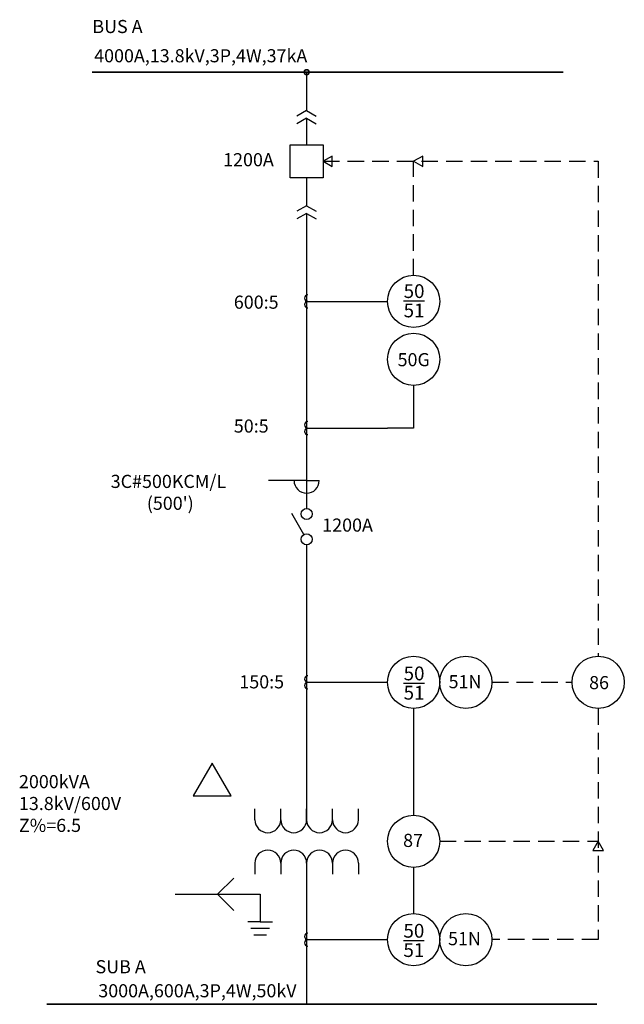
# Model space of a CAD drawing. Units: millimetres. Extents: x 325 to 734, y 204 to 452.
# Tile 1 of 1: x 642.1 to 734.2, y 301.6 to 451.7. Entities that reach past the tile are written whole.
import ezdxf

# ---------------------------------------------------------------- set-up
doc = ezdxf.new("R2010")
doc.units = ezdxf.units.MM
doc.header["$MEASUREMENT"] = 0
doc.linetypes.add('HIDDENX2', pattern=[0.75, 0.5, -0.25])
for name, color, linetype, lineweight in [('E-ANNO-TEXT', 7, 'Continuous', 25), ('E-CTRL-RLAY', 5, 'Continuous', 30), ('E-CTRL-SENS', 5, 'Continuous', 25), ('E-CTRL-SYMB', 3, 'Continuous', 30), ('E-CTRL-TRIP', 1, 'HIDDENX2', 30), ('E-POWR-BUSB', 3, 'Continuous', 35), ('E-POWR-CABL', 5, 'Continuous', 30), ('E-POWR-CONN', 7, 'Continuous', 30), ('E-POWR-CT', 5, 'Continuous', 30), ('E-POWR-FEED', 3, 'Continuous', 30), ('E-POWR-IDEN', 6, 'Continuous', 25), ('E-POWR-SWGR', 6, 'Continuous', 30), ('E-POWR-XFMR', 6, 'Continuous', 30)]:
    doc.layers.add(name, color=color, linetype=linetype, lineweight=lineweight)
doc.styles.get("Standard").update_dxf_attribs({"font": 'arial.ttf'})

# ---------------------------------------------------------------- blocks, each defined once
blk = doc.blocks.new('DRAWOUT-CONTACT')
for p, q in [((0, 0), (-1.47, -0.85)), ((0, 0), (1.47, -0.85)), ((0, -1.17), (-1.47, -2.01)), ((0, -1.17), (1.47, -2.01))]:
    blk.add_line(p, q)
blk = doc.blocks.new('XFMR-WINDING')
for p, q in [((-7.89, 0), (-7.89, 1.68)), ((-3.95, 0), (-3.95, 1.68)), ((0, 0), (0, 1.68)), ((3.95, 0), (3.95, 1.68)), ((7.89, 0), (7.89, 1.68))]:
    blk.add_line(p, q)
for centre in [(-5.92, 0), (-1.97, 0), (1.97, 0), (5.92, 0)]:
    blk.add_arc(centre, 1.97, 180, 0)
blk = doc.blocks.new('CURRENT-TRANSFORMER')
for centre in [(0.19, 0.5), (0.19, -0.5)]:
    blk.add_arc(centre, 0.501, 90, 270)
blk = doc.blocks.new('PROTECTIVE-RELAY')
blk.add_circle((0, 0), 3.98)
blk = doc.blocks.new('TRIP-ARROW')
blk.add_lwpolyline([(0.79, -1.38), (0, 0), (-0.79, -1.38)], close=True)

msp = doc.modelspace()

# ---------------------------------------------------------------- linework, layer by layer
at = {"layer": 'E-CTRL-SENS'}
for p, q in [((685.83, 408.77), (698.14, 408.77)), ((702.13, 395.94), (702.13, 389.45)), ((685.83, 389.45), (698.14, 389.45)), ((702.13, 389.45), (698.14, 389.45)), ((685.83, 350.69), (698.14, 350.69)), ((702.13, 346.71), (702.13, 330.42)), ((702.13, 322.45), (702.13, 315.44)), ((685.83, 311.45), (698.14, 311.45))]:
    msp.add_line(p, q, dxfattribs=at)
at = {"layer": 'E-CTRL-TRIP', "ltscale": 5}
for p, q in [((688.33, 430.13), (730.25, 430.13)), ((702.13, 412.75), (702.13, 430.13)), ((730.25, 430.13), (730.25, 354.68)), ((714.08, 350.69), (726.26, 350.69)), ((730.25, 346.71), (730.25, 311.45)), ((706.11, 326.44), (730.25, 326.44)), ((730.25, 311.45), (714.08, 311.45))]:
    msp.add_line(p, q, dxfattribs=at)
at = {"layer": 'E-POWR-BUSB'}
for p, q in [((676.68, 443.72), (653.14, 443.72)), ((676.68, 443.72), (694.99, 443.72)), ((694.99, 443.72), (724.93, 443.72)), ((661.25, 301.59), (646.23, 301.59)), ((661.25, 301.59), (730.04, 301.59))]:
    msp.add_line(p, q, dxfattribs=at)
at = {"layer": 'E-POWR-BUSB', "const_width": 0.25}
msp.add_lwpolyline([(685.46, 443.72, 1), (686.21, 443.72, 1)], format="xyb", close=True, dxfattribs=at)
at = {"layer": 'E-POWR-CABL'}
for q in [(680.01, 381.44), (687.76, 381.44)]:
    msp.add_line((685.83, 381.44), q, dxfattribs=at)
msp.add_arc((685.83, 381.44), 1.92, 180, 0, dxfattribs=at)
at = {"layer": 'E-POWR-CONN'}
for p, q in [((672.26, 318.36), (674.74, 320.83)), ((665.78, 318.36), (678.75, 318.36)), ((672.26, 318.36), (674.74, 315.89)), ((678.75, 318.36), (678.75, 314.18)), ((678.75, 314.18), (676.88, 314.18)), ((678.75, 314.18), (680.62, 314.18)), ((677.34, 313.18), (680.17, 313.18)), ((677.79, 312.18), (679.71, 312.18))]:
    msp.add_line(p, q, dxfattribs=at)
msp.add_lwpolyline([(671.42, 338.38), (668.52, 333.36), (674.32, 333.36)], close=True, dxfattribs=at)
at = {"layer": 'E-POWR-FEED'}
for p, q in [((685.83, 443.72), (685.83, 437.85)), ((685.83, 436.68), (685.83, 432.63)), ((685.83, 427.63), (685.83, 423.35)), ((685.83, 422.18), (685.83, 389.45)), ((685.83, 389.45), (685.83, 377.21)), ((685.83, 371.65), (685.83, 329.73)), ((685.83, 323.12), (685.83, 301.59))]:
    msp.add_line(p, q, dxfattribs=at)
at = {"layer": 'E-POWR-SWGR'}
msp.add_line((685.41, 373.23), (683.57, 376.41), dxfattribs=at)
msp.add_lwpolyline([(683.33, 432.63), (688.33, 432.63), (688.33, 427.63), (683.33, 427.63)], close=True, dxfattribs=at)
for centre in [(685.83, 376.36), (685.83, 372.5)]:
    msp.add_circle(centre, 0.844, dxfattribs=at)

# ---------------------------------------------------------------- block references
at = {"layer": 'E-CTRL-RLAY'}
for p in [(702.13, 408.77), (702.13, 399.93), (702.13, 350.69), (710.09, 350.69), (730.25, 350.69), (702.13, 326.44), (702.13, 311.45), (710.09, 311.45)]:
    msp.add_blockref('PROTECTIVE-RELAY', p, dxfattribs=at)
at = {"layer": 'E-CTRL-SYMB'}
for p, rotation in [((688.33, 430.13), 90.00000000000126), ((702.13, 430.13), 90.00000000000246)]:
    msp.add_blockref('TRIP-ARROW', p, dxfattribs=dict(at, rotation=rotation))
msp.add_blockref('TRIP-ARROW', (730.25, 326.44), dxfattribs=at)
at = {"layer": 'E-POWR-CT'}
for p in [(685.83, 408.77), (685.83, 389.45), (685.83, 350.69), (685.83, 311.45)]:
    msp.add_blockref('CURRENT-TRANSFORMER', p, dxfattribs=at)
at = {"layer": 'E-POWR-SWGR'}
for p in [(685.83, 437.85), (685.83, 423.35)]:
    msp.add_blockref('DRAWOUT-CONTACT', p, dxfattribs=at)
at = {"layer": 'E-POWR-XFMR'}
msp.add_blockref('XFMR-WINDING', (685.83, 329.73), dxfattribs=at)
at = {"layer": 'E-POWR-XFMR', "rotation": 180}
msp.add_blockref('XFMR-WINDING', (685.83, 323.12), dxfattribs=at)

# ---------------------------------------------------------------- texts
at = {"layer": 'E-ANNO-TEXT', "attachment_point": 1}
for s, width, insert, char_height in [('4000A,13.8kV,3P,4W,37kA', 14.1582, (653.46, 447.22), 2), ('1200A', 14.1582, (673.11, 431.37), 2), ('\\A1;{\\H0.7x;\\S50/51;}', 3.2823, (700.61, 411.38), 3), ('600:5', 14.1582, (674.74, 409.65), 2), ('\\A1;{\\H1x;50G}', 3.2823, (699.69, 400.88), 2), ('50:5', 14.1582, (674.74, 390.76), 2), ("3C#500KCM/L\\P         (500')", 14.1582, (655.98, 382.32), 2), ('1200A', 14.1582, (688.21, 375.66), 2), ('\\A1;{\\H0.7x;\\S50/51;}', 3.2823, (700.61, 353.09), 3), ('150:5', 14.1582, (675.58, 351.76), 2), ('\\A1;51N', 3.2823, (707.46, 351.78), 2), ('\\A1;86', 3.2823, (728.87, 351.64), 2), ('2000kVA\\P13.8kV/600V\\PZ%=6.5', 14.1582, (642, 336.54), 2), ('\\A1;87', 3.2823, (700.53, 327.58), 2), ('\\A1;{\\H0.7x;\\S50/51;}', 3.2823, (700.58, 313.85), 3), ('\\A1;51N', 3.2823, (707.38, 312.6), 2), ('3000A,600A,3P,4W,50kV', 14.1582, (654.09, 304.66), 2)]:
    msp.add_mtext_dynamic_manual_height_columns(s, width=width, gutter_width=1, heights=[0], dxfattribs=dict(at, insert=insert, char_height=char_height))
at = {"layer": 'E-POWR-IDEN', "char_height": 2, "attachment_point": 1}
for s, insert in [('BUS A', (653.18, 451.68)), ('SUB A', (653.67, 308.32))]:
    msp.add_mtext_dynamic_manual_height_columns(s, width=14.1582, gutter_width=1, heights=[0], dxfattribs=dict(at, insert=insert))

doc.saveas('drawing.dxf')
